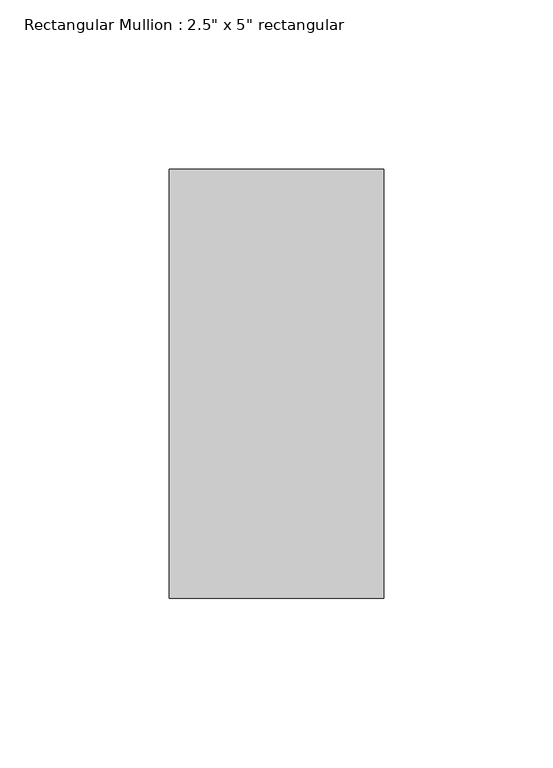
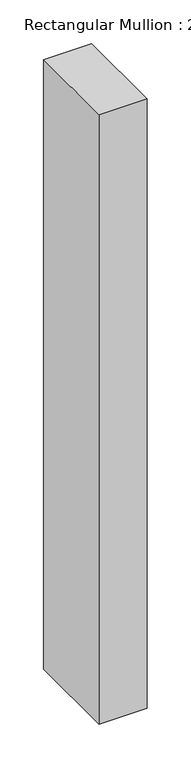
"""IFC4 building model written with IfcOpenShell, lengths in millimetres: member geometry."""

from ifc_helpers import new_model, si_unit, frame, origin, place, context, project, spatial, polyline, outline, extrude, source, transform, mapped, element, save


def member_d2e7e466(model_context):
    return source(origin(), model_context, "Body", "SweptSolid", [
        extrude(outline(polyline([(0.0, 63.5), (0.0, -63.5), (-63.5, -63.5), (-63.5, 63.5), (0.0, 63.5)])), frame((0.0, 0.0, -850.9), z_axis=(0.0, 0.0, 1.0), x_axis=(1.0, 0.0, 0.0)), (0.0, 0.0, 1.0), 850.9),
    ])


if __name__ == "__main__":
    model = new_model("IFC4")
    model_context = context("Model", 3, world=origin())
    ifc_project = project(units=[si_unit("LENGTHUNIT", "METRE", prefix="MILLI")], contexts=[model_context])
    site = spatial("IfcSite", under=ifc_project)
    building = spatial("IfcBuilding", under=site)
    placement = place(None, origin())
    member_shape = member_d2e7e466(model_context)
    element("IfcMember", 1, ObjectType="Rectangular Mullion : 2.5\" x 5\" rectangular", at=placement, inside=building, context=model_context, shape_type="MappedRepresentation", body=[
        mapped(member_shape, transform((0.0, 0.0, 0.0), x_axis=(1.0, 0.0, 0.0), y_axis=(0.0, 1.0, 0.0), z_axis=(0.0, 0.0, 1.0))),
    ])
    save(model, "model.ifc")

# Revit data of these elements
# Type "Rectangular Mullion : 2.5\" x 5\" rectangular"
#   built-in parameter 1007304 = 0.416667 (stored number, unit not read)
#   built-in parameter 1007301 = 0.104167 (stored number, unit not read)
#   built-in parameter 1007300 = 0.104167 (stored number, unit not read)
# Element 1 (IfcMember, "Rectangular Mullion : 2.5\" x 5\" rectangular")
#   Materials on its faces: "Aluminum"
# Materials
#   "Aluminum": class "Metal", colour RGB 247 247 247, transparency 0, Description = "Aluminum 6061", Cost = 0
